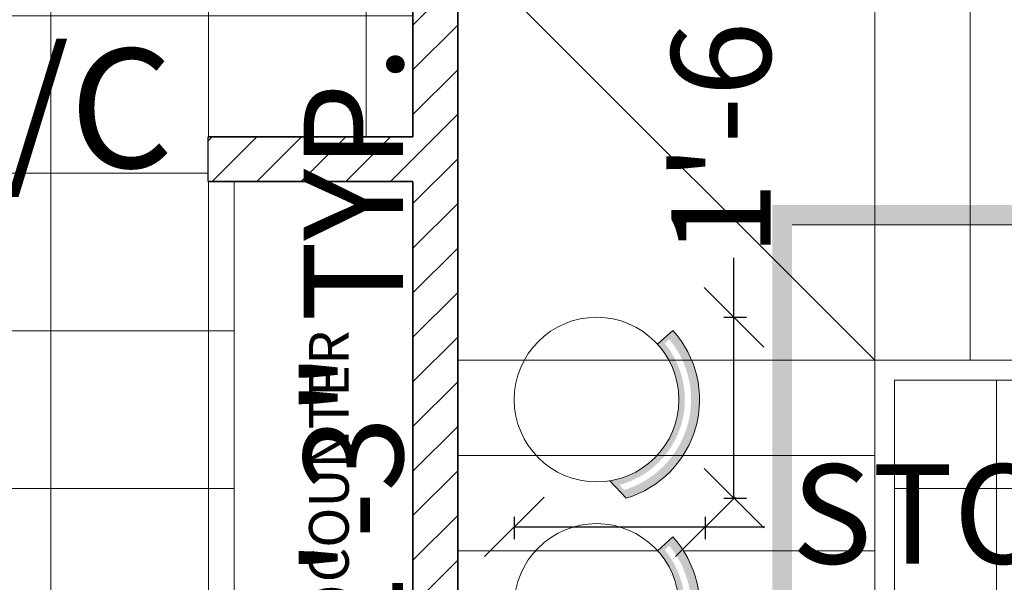
# Model space of a CAD drawing. Units: inches. Extents: x 2036 to 2670, y 319 to 920.
# Tile 9 of 15: x 2251 to 2350, y 784 to 841. Entities that reach past the tile are written whole.
import ezdxf

# ---------------------------------------------------------------- set-up
doc = ezdxf.new("R2010")
doc.units = ezdxf.units.IN
for name, color, linetype, lineweight in [('A-ANNO-DIMS', 2, 'Continuous', 18), ('A-ANNO-SYMB', 7, 'Continuous', 18), ('A-ANNO-SYMB-PATT', 7, 'Continuous', 13), ('A-ANNO-TEXT', 7, 'Continuous', 18), ('A-CASE', 7, 'Continuous', 18), ('A-DOOR', 3, 'Continuous', 25), ('A-FLOR-PATT', 8, 'Continuous', 9), ('A-FLOR-STRS', 7, 'Continuous', 18), ('A-FURN', 8, 'Continuous', 18), ('A-WALL', 7, 'Continuous', 35)]:
    doc.layers.add(name, color=color, linetype=linetype, lineweight=lineweight)
doc.layers.add('A-FURN-PATT', color=242, linetype='Continuous', lineweight=9, true_color=0xcd2027)
doc.layers.add('A-WALL-PATT', color=52, linetype='Continuous', lineweight=13, true_color=0xc8c92d)
doc.styles.get("Standard").update_dxf_attribs({"font": 'arial.ttf'})
doc.dimstyles.new('ISO-25', dxfattribs={"dimtxt": 10, "dimasz": 6, "dimexe": 1.25, "dimexo": 0.625, "dimtad": 0, "dimdec": 1, "dimlunit": 3, "dimtxsty": 'Standard', "dimblk": 'OBLIQUE', "dimcen": 2.5, "dimclrd": 94, "dimclre": 94, "dimclrt": 1, "dimadec": 0, "dimazin": 0, "dimtfac": 1, "dimtdec": 1, "dimtmove": 0, "dimatfit": 3, "dimfxl": 1, "dimfxlon": 1, "dimarcsym": 0})

# ---------------------------------------------------------------- blocks, each defined once
blk = doc.blocks.new('STOOL-COUNTER')
for p, q in [((14.44209721263451, 15.49845302218841), (15.97906463249819, 16.89025742639614)), ((16.25127518254248, 16.57729449613657), (16.25742551333951, 16.5828639424235)), ((9.61939974663892, 1.743797943406207), (11.27062915654505, 0.0001860092081643))]:
    blk.add_line(p, q)
blk.add_circle((8.294227533182038, 9.93123540535771), 8.29398659202474)
blk.add_arc((8.294227533182038, 9.93123540535771), 10.36748324003093, 286.6838234776646, 42.16248726182812)
blk = doc.blocks.new('_Oblique')
at = {"color": 0, "linetype": 'ByBlock', "lineweight": -2}
blk.add_line((-0.5, -0.5), (0.5, 0.5), dxfattribs=at)
blk = doc.blocks.new('*D23')
at = {"layer": 'A-ANNO-DIMS', "color": 94, "lineweight": -2, "transparency": 16777216}
for p, q in [((2286.028582728119, 660.1846446428973), (2286.028582728119, 666.1846446428973)), ((2285.02858272812, 660.1846446428973), (2287.27858272812, 660.1846446428973)), ((2286.028582728119, 633.1846547235), (2286.028582728119, 660.1846446428973)), ((2285.02858272812, 633.1846547235), (2287.27858272812, 633.1846547235))]:
    blk.add_line(p, q, dxfattribs=at)
at = {"layer": 'Defpoints', "color": 0, "transparency": 16777216}
for p in [(2281.978584240209, 660.1846446428973), (2286.028582728119, 660.1846446428973), (2281.978584240209, 633.1846547235)]:
    blk.add_point(p, dxfattribs=at)
at = {"layer": 'A-ANNO-DIMS', "color": 94, "lineweight": -2, "transparency": 16777216, "xscale": 6, "yscale": 6, "zscale": 6}
for p, rotation in [((2286.028582728119, 660.1846446428973), 90), ((2286.028582728119, 633.1846547235), 270)]:
    blk.add_blockref('_Oblique', p, dxfattribs=dict(at, rotation=rotation))
at = {"layer": 'A-ANNO-DIMS', "color": 1, "transparency": 16777216, "insert": (2286.028582728119, 755.2407496906455), "char_height": 10, "attachment_point": 5, "rotation": 90}
blk.add_mtext('ROCKING CHAIR 2\'-3" TYP.', dxfattribs=at)
blk = doc.blocks.new('*D27')
at = {"layer": 'A-ANNO-DIMS', "color": 94, "lineweight": -2, "transparency": 16777216}
for p, q in [((2300.931240941157, 790.9031204416938), (2300.931240941157, 788.6531204416938)), ((2320.167405879669, 790.9031204416938), (2320.167405879669, 788.6531204416938)), ((2300.931240941157, 789.9031204416937), (2320.167405879669, 789.9031204416937)), ((2320.167405879669, 789.9031204416937), (2326.167405879669, 789.9031204416937))]:
    blk.add_line(p, q, dxfattribs=at)
at = {"layer": 'Defpoints', "color": 0, "transparency": 16777216}
for p in [(2300.931240941157, 792.7885451824704), (2320.167405879669, 792.7885451824704), (2320.167405879669, 789.9031204416937)]:
    blk.add_point(p, dxfattribs=at)
at = {"layer": 'A-ANNO-DIMS', "color": 94, "lineweight": -2, "transparency": 16777216, "xscale": 6, "yscale": 6, "zscale": 6, "rotation": 180}
blk.add_blockref('_Oblique', (2300.931240941157, 789.9031204416937), dxfattribs=at)
at = {"layer": 'A-ANNO-DIMS', "color": 94, "lineweight": -2, "transparency": 16777216, "xscale": 6, "yscale": 6, "zscale": 6}
blk.add_blockref('_Oblique', (2320.167405879669, 789.9031204416937), dxfattribs=at)
at = {"layer": 'A-ANNO-DIMS', "color": 1, "transparency": 16777216, "insert": (2382.86334721664, 789.9031204416937), "char_height": 10, "attachment_point": 5}
blk.add_mtext('STOOL 1\'-7" TYP.', dxfattribs=at)
blk = doc.blocks.new('*D28')
at = {"layer": 'A-ANNO-DIMS', "color": 94, "lineweight": -2, "transparency": 16777216}
for p, q in [((2323.052830620447, 811.0135811706456), (2323.052830620447, 817.0135811706456)), ((2322.052830620447, 811.0135811706456), (2324.302830620447, 811.0135811706456)), ((2323.052830620447, 792.7885451824709), (2323.052830620447, 811.0135811706456)), ((2322.052830620447, 792.7885451824709), (2324.302830620447, 792.7885451824709))]:
    blk.add_line(p, q, dxfattribs=at)
at = {"layer": 'Defpoints', "color": 0, "transparency": 16777216}
for p in [(2320.167405879669, 811.0135811706456), (2323.052830620447, 811.0135811706456), (2320.167405879669, 792.7885451824709)]:
    blk.add_point(p, dxfattribs=at)
at = {"layer": 'A-ANNO-DIMS', "color": 94, "lineweight": -2, "transparency": 16777216, "xscale": 6, "yscale": 6, "zscale": 6}
for p, rotation in [((2323.052830620447, 811.0135811706456), 90), ((2323.052830620447, 792.7885451824709), 270)]:
    blk.add_blockref('_Oblique', p, dxfattribs=dict(at, rotation=rotation))
at = {"layer": 'A-ANNO-DIMS', "color": 1, "transparency": 16777216, "insert": (2323.052830620447, 847.6454024530459), "char_height": 10, "attachment_point": 5, "rotation": 90}
blk.add_mtext('1\'-6" TYP.', dxfattribs=at)
blk = doc.blocks.new('*D58')
at = {"layer": 'A-ANNO-DIMS', "color": 94, "lineweight": -2, "transparency": 16777216}
for p, q in [((2224.735119, 436.334645), (2224.735119, 434.0846449999999)), ((2270.113432, 436.334645), (2270.113432, 434.0846449999999)), ((2224.735119, 435.334645), (2270.113432, 435.334645)), ((2270.113432, 435.334645), (2276.113432, 435.334645))]:
    blk.add_line(p, q, dxfattribs=at)
at = {"layer": 'Defpoints', "color": 0, "transparency": 16777216}
for p in [(2224.735119, 824.684645), (2270.113432, 824.684645), (2270.113432, 435.334645)]:
    blk.add_point(p, dxfattribs=at)
at = {"layer": 'A-ANNO-DIMS', "color": 94, "lineweight": -2, "transparency": 16777216, "xscale": 6, "yscale": 6, "zscale": 6, "rotation": 180}
blk.add_blockref('_Oblique', (2224.735119, 435.334645), dxfattribs=at)
at = {"layer": 'A-ANNO-DIMS', "color": 94, "lineweight": -2, "transparency": 16777216, "xscale": 6, "yscale": 6, "zscale": 6}
blk.add_blockref('_Oblique', (2270.113432, 435.334645), dxfattribs=at)
at = {"layer": 'A-ANNO-DIMS', "color": 1, "transparency": 16777216, "insert": (2301.677040458391, 435.334645), "char_height": 10, "attachment_point": 5}
blk.add_mtext('3\'-9 1/2"', dxfattribs=at)

msp = doc.modelspace()

# ---------------------------------------------------------------- hatches: boundary and pattern name
at = {"layer": 'A-ANNO-SYMB-PATT'}
h = msp.add_hatch(color=256, dxfattribs=at)
h.dxf.hatch_style = 1
h.paths.add_polyline_path([(2406.873099182944, 822.3319931427415), (2326.913490001141, 822.3319931427415), (2326.913490001141, 772.4185847172232), (2322.238393735226, 772.4185847172232), (2328.913490001141, 764.3321655646498), (2328.913490001141, 772.4185847172232), (2328.913490001141, 820.3319931427413), (2404.873099182943, 820.3319931427413), (2404.873099182944, 731.1997691085871), (2406.873099182944, 731.1997691085871)])
at = {"layer": 'A-FLOR-PATT'}
h = msp.add_hatch(dxfattribs=at)
h.set_pattern_fill('ANSI31', color=256, scale=5, angle=135)
h.set_pattern_definition([(180, (0, 0), (-1.8e-15, -15.875), [])])
h.paths.add_polyline_path([(2290.73511852215, 659.6846447234993), (2158.73511852215, 659.6846447234993), (2158.73511852215, 582.5347262125274), (2158.73511852215, 545.5097979180838), (2158.73511852215, 503.6846447234993), (2426.735118522151, 503.6846447234993), (2426.735118522151, 614.6846447234993), (2426.735118522151, 623.6846447234993), (2426.735118522151, 628.1846447234993), (2431.235118522151, 628.1846447234993), (2431.235118522151, 623.6846447234993), (2438.735118522151, 623.6846447234993), (2438.735118522151, 619.1846447234993), (2574.394321277629, 619.1846447234993), (2574.394321277629, 623.7052101185), (2586.394321277629, 623.7052101185), (2586.394321277629, 619.1846447234993), (2603.735118522151, 619.1846447234993), (2603.735118522151, 824.6846447234993), (2431.73511852215, 824.6846447234993), (2431.73511852215, 746.0911818027907), (2439.235118522151, 746.0911818027907), (2439.235118522151, 737.0911818027907), (2431.73511852215, 737.0911818027907), (2431.73511852215, 659.6846447234992), (2427.235118522151, 659.6846447234992), (2427.235118522151, 739.4846447234991), (2383.235118522151, 739.4846447234991), (2383.23511852215, 804.6846447234994), (2339.235118522151, 804.6846447234994), (2339.235118522151, 749.0846447234992), (2295.235118522151, 749.084644723499), (2295.235118522151, 737.6459187756934), (2295.267038589669, 737.6459187756934), (2295.267038589669, 728.6459187756934), (2295.213454263402, 728.6459187756934, -0.5864181262682077), (2272.735118522151, 728.6846447234993), (2272.735118522151, 824.6846447234994), (2270.11343239043, 824.6846447234994), (2270.11343239043, 829.1846447234994), (2290.73511852215, 829.1846447234993), (2290.73511852215, 848.663139280863), (2283.207837384491, 848.663139280863), (2283.207837384491, 857.663139280863), (2289.735118522151, 857.663139280863), (2289.735118522151, 874.6846447234994), (2158.73511852215, 874.6846447234993), (2158.73511852215, 852.8142946291669), (2161.73511852215, 852.8142946291669), (2161.73511852215, 843.8142946291669), (2158.73511852215, 843.8142946291669), (2158.73511852215, 829.1846447234993), (2224.73511852215, 829.1846447234993), (2224.73511852215, 800.6846447234994), (2182.735118522151, 800.6846447234994), (2182.735118522151, 733.4146909245898), (2158.73511852215, 733.4146909245898), (2158.73511852215, 728.6846447234993), (2235.235118522151, 728.6846447234993), (2235.235118522151, 714.8073923633797), (2230.735118522151, 714.8073923633797), (2230.735118522151, 724.1846447234991), (2158.73511852215, 724.1846447234993), (2158.73511852215, 664.1846447234993), (2230.735118522151, 664.1846447234993), (2230.735118522151, 678.8073923633796), (2235.235118522151, 678.8073923633796), (2235.235118522151, 664.1846447234993), (2290.73511852215, 664.1846447234993)])
h.paths.add_polyline_path([(2309.267682807548, 612.1195713103912), (2309.267682807548, 603.1195713103912), (2297.267682807548, 603.1195713103912), (2297.267682807548, 612.1195713103912)], flags=16)
h.paths.add_polyline_path([(2280.116432231614, 639.1101421987634), (2280.261038064034, 638.1846547234999, -0.4142135623730951), (2279.261038064034, 637.1846547234999), (2278.761038064034, 637.1846547234999), (2279.261038064034, 633.1846547234999), (2277.761038064034, 633.1846547234999), (2277.261038064034, 637.1846547234999), (2269.761038064034, 637.1846547234999), (2262.261038064034, 637.1846547234999), (2261.761038064034, 633.1846547234999), (2260.261038064034, 633.1846547234999), (2260.761038064034, 637.1846547234999), (2260.261038064034, 637.1846547234999, -0.4142135623730951), (2259.261038064034, 638.1846547234999), (2259.405649624543, 639.1101427248512, -0.5411643393254109), (2257.761038870006, 641.1846576787281), (2260.761038064034, 652.1846447234999), (2261.448547850994, 652.1846447234999), (2261.52666276384, 652.6846447234999), (2262.761038064034, 652.6846447234999), (2262.249174101338, 655.2439645369782, 0.0019132646615086), (2261.761062671999, 655.1846078115532), (2259.76103814896, 658.1846445961108, -0.1500000140127399), (2279.761037979108, 658.184644596111), (2277.761013456069, 655.1846078115531, 0.0019132646615084), (2277.27290202673, 655.243964536978), (2276.761038064034, 652.6846447234999), (2277.995414002001, 652.6846447234999), (2278.073538681693, 652.1846447234999), (2278.761038064034, 652.1846447234999), (2281.761037258062, 641.1846576787256, -0.5411631634674846)], flags=16)
h.paths.add_polyline_path([(2245.983724681685, 639.1101421987634), (2246.128330514105, 638.1846547234998, -0.4142135623730951), (2245.128330514105, 637.1846547234996), (2244.628330514105, 637.1846547234996), (2245.128330514105, 633.1846547234996), (2243.628330514105, 633.1846547234996), (2243.128330514105, 637.1846547234996), (2235.628330514105, 637.1846547234996), (2228.128330514104, 637.1846547234996), (2227.628330514105, 633.1846547234996), (2226.128330514105, 633.1846547234996), (2226.628330514105, 637.1846547234996), (2226.128330514105, 637.1846547234996, -0.4142135623730951), (2225.128330514105, 638.1846547234998), (2225.272942074614, 639.1101427248511, -0.5411643393254109), (2223.628331320076, 641.184657678728), (2226.628330514105, 652.1846447234998), (2227.315840301064, 652.1846447234998), (2227.393955213911, 652.6846447234998), (2228.628330514105, 652.6846447234998), (2228.116466551409, 655.243964536978, 0.0019132646615086), (2227.628355122069, 655.1846078115532), (2225.628330599031, 658.1846445961108, -0.1500000140127405), (2245.628330429179, 658.1846445961108), (2243.62830590614, 655.184607811553, 0.0019132646615084), (2243.140194476801, 655.2439645369778), (2242.628330514105, 652.6846447234998), (2243.862706452072, 652.6846447234998), (2243.940831131764, 652.1846447234998), (2244.628330514105, 652.1846447234998), (2247.628329708133, 641.1846576787256, -0.5411631634675002)], flags=16)
h.paths.add_polyline_path([(2351.589714523122, 515.1547705889745, -0.151947809280591), (2279.589707523122, 515.1547621898734), (2279.589707523122, 537.684644723502), (2273.589707523122, 537.684644723502), (2273.589707523122, 511.6846368176175, 0.1904762075443491), (2357.589714523122, 511.6846553964427), (2357.589714523122, 537.684644723502), (2351.589714523122, 537.684644723502)])
h.paths.add_polyline_path([(2327.589707523122, 536.1267447235019), (2327.589714897934, 517.0665447235019), (2303.58971014831, 517.0665447235019), (2303.589717523122, 536.1267447235019)], flags=16)
h.paths.add_polyline_path([(2213.4008319258, 639.1101421987634), (2213.545437758219, 638.1846547234998, -0.4142135623730951), (2212.545437758219, 637.1846547234996), (2212.045437758219, 637.1846547234996), (2212.545437758219, 633.1846547234996), (2211.045437758219, 633.1846547234996), (2210.545437758219, 637.1846547234996), (2203.045437758219, 637.1846547234996), (2195.545437758219, 637.1846547234996), (2195.045437758219, 633.1846547234996), (2193.545437758219, 633.1846547234996), (2194.045437758219, 637.1846547234996), (2193.545437758219, 637.1846547234996, -0.4142135623730951), (2192.545437758219, 638.1846547234998), (2192.690049318728, 639.1101427248511, -0.5411643393254677), (2191.045438564191, 641.1846576787283), (2194.045437758219, 652.1846447234998), (2194.732947545178, 652.1846447234998), (2194.811062458025, 652.6846447234998), (2196.045437758219, 652.6846447234998), (2195.533573795524, 655.243964536978, 0.0019132646615086), (2195.045462366184, 655.1846078115532), (2193.045437843145, 658.1846445961108, -0.1500000140127405), (2213.045437673293, 658.1846445961108), (2211.045413150255, 655.184607811553, 0.0019132646615084), (2210.557301720915, 655.2439645369778), (2210.045437758219, 652.6846447234998), (2211.279813696187, 652.6846447234998), (2211.357938375878, 652.1846447234998), (2212.045437758219, 652.1846447234998), (2215.045436952248, 641.1846576787256, -0.541163163467504)], flags=16)
h.paths.add_polyline_path([(2368.579245727136, 538.0174860170698), (2370.522614835591, 538.0174860170698), (2371.170404538409, 532.8351683945237), (2380.887250080682, 532.8351683945237), (2390.604095622956, 532.8351683945237), (2391.251885325774, 538.0174860170698), (2393.195254434229, 538.0174860170698), (2392.547464731411, 532.8351683945237), (2380.887250080682, 532.8351683945237), (2368.579245727136, 532.8351683945237, 0.4142135623730823), (2367.283666321499, 531.5395889888874), (2367.471014659917, 530.3405464757611, -0.4833518268794939), (2369.227035511853, 527.6528503215334), (2371.818194241227, 513.4014902657708), (2370.117745471103, 513.4014902657708), (2370.218962197183, 512.7537005629525), (2391.555537137895, 512.7537005629525), (2391.656741210253, 513.4014902657708), (2389.956305920138, 513.4014902657708), (2392.547464649512, 527.6528503215332, -1.387427444475197), (2396.43420190412, 527.6528469432474), (2392.547464731411, 513.4014902657708), (2391.656741210253, 513.4014902657708), (2391.555537137895, 512.7537005629525), (2389.30851621732, 512.7537005629525), (2389.996735292977, 509.3669642787241, 0.003795645225288), (2391.251853444202, 509.5147998712193), (2393.843044027018, 505.6280139969943, -0.1500000140127354), (2367.931456134346, 505.6280139969944), (2370.522646717163, 509.5147998712195, 0.0039006605371613), (2371.812521455224, 509.3631450934526), (2372.465983944045, 512.7537005629525), (2370.218962197183, 512.7537005629525), (2370.117745471103, 513.4014902657708), (2369.227035429954, 513.4014902657708), (2365.340298257246, 527.6528469432453, -0.5411631634679974), (2367.471014659917, 530.3405464757611), (2367.283666321499, 531.5395889888874, -0.4142135623730824), (2368.579245727136, 532.8351683945237), (2369.227035429954, 532.8351683945237)])
h.paths.add_polyline_path([(2266.737911501414, 538.0174860170694), (2266.090121798596, 532.8351683945236), (2254.429907147867, 532.8351683945236), (2242.121902794321, 532.8351683945235, 0.4142135623730823), (2240.826323388684, 531.539588988887), (2241.013671727102, 530.3405464757608, -0.4833518268795056), (2242.769692579038, 527.652850321533), (2245.360851308412, 513.4014902657705), (2243.660402538288, 513.4014902657705), (2243.761619264368, 512.7537005629522), (2265.09819420508, 512.7537005629522), (2265.199398277438, 513.4014902657703), (2263.498962987323, 513.4014902657703), (2266.090121716697, 527.6528503215327, -1.387427444474997), (2269.976858971305, 527.6528469432478), (2266.090121798596, 513.4014902657703), (2265.199398277438, 513.4014902657703), (2265.09819420508, 512.7537005629522), (2262.851173284504, 512.7537005629522), (2263.539392360161, 509.3669642787239, 0.0037956452252879), (2264.794510511388, 509.5147998712191), (2267.385701094204, 505.628013996994, -0.1500000140127357), (2241.474113201531, 505.6280139969941), (2244.065303784347, 509.5147998712193, 0.0039006605371612), (2245.355178522409, 509.3631450934523), (2246.00864101123, 512.7537005629522), (2243.761619264368, 512.7537005629522), (2243.660402538288, 513.4014902657705), (2242.769692497139, 513.4014902657705), (2238.88295532443, 527.6528469432458, -0.541163163467894), (2241.013671727102, 530.3405464757608), (2240.826323388684, 531.539588988887, -0.4142135623730824), (2242.121902794321, 532.8351683945235), (2242.769692497139, 532.8351683945235), (2242.121902794321, 538.0174860170694), (2244.065271902775, 538.0174860170694), (2244.713061605594, 532.8351683945236), (2254.429907147867, 532.8351683945236), (2264.146752690141, 532.8351683945236), (2264.794542392959, 538.0174860170694)])
h.paths.add_polyline_path([(2185.23510852215, 620.3554545661904), (2185.23510852215, 618.8554545661904), (2181.23510852215, 618.3554545661904), (2181.23510852215, 610.8554545661904), (2181.23510852215, 603.3554545661904), (2185.23510852215, 602.8554545661904), (2185.23510852215, 601.3554545661905), (2181.23510852215, 601.8554545661904), (2181.23510852215, 601.3554545661905, -0.4142135623730951), (2180.23510852215, 600.3554545661905), (2179.309620520799, 600.5000661266993, -0.5411643393248329), (2177.235105566925, 598.8554553721619), (2166.23511852215, 601.8554545661904), (2166.23511852215, 602.5429643531498), (2165.73511852215, 602.6210792659967), (2165.73511852215, 603.8554545661904), (2163.175798708671, 603.3435906034947, 0.0019132646615093), (2163.235155434097, 602.8554791741547), (2160.235118649539, 600.8554546511162, -0.1500000140127393), (2160.235118649539, 620.8554544812645), (2163.235155434097, 618.855429958226, 0.0019132646615086), (2163.175798708672, 618.3673185288861), (2165.73511852215, 617.8554545661905), (2165.73511852215, 619.0898305041582), (2166.23511852215, 619.167955183849), (2166.23511852215, 619.8554545661904), (2177.235105566925, 622.855453760219, -0.5411631634675461), (2179.309621046886, 621.2108487337705), (2180.23510852215, 621.3554545661905, -0.4142135623730951), (2181.23510852215, 620.3554545661904), (2181.23510852215, 619.8554545661904)])
h.paths.add_polyline_path([(2470.924455674587, 676.0076055808825), (2470.924455674587, 806.1287861477749), (2568.515288238047, 806.1287861477749), (2568.515288238047, 676.0076055808825)], flags=16)
h.paths.add_polyline_path([(2177.737763186158, 677.4877546326836), (2161.903034523561, 677.4877546326836), (2161.903034523561, 705.8482879805396), (2177.737763186158, 705.8482879805396)], flags=16)
h.paths.add_polyline_path([(2176.737763186158, 678.4877546326836), (2162.903034523562, 678.4877546326836), (2162.903034523562, 704.8482879805395), (2176.737763186158, 704.8482879805395)], flags=0)
h.paths.add_polyline_path([(2175.006477017632, 686.4819431438401), (2172.932045752523, 686.4819431438401), (2172.932045752523, 690.6308056740573), (2170.857614487415, 690.6308056740573), (2170.857614487415, 686.4819431438401), (2164.634320692089, 686.4819431438401), (2164.634320692089, 688.556374408949), (2166.708751957198, 688.5563744089487), (2168.783183222306, 688.5563744089487), (2168.783183222306, 690.6308056740573), (2164.634320692089, 690.6308056740575), (2164.634320692089, 696.8540994693836), (2166.708751957198, 696.8540994693833), (2166.708751957198, 692.7052369391664), (2168.783183222306, 692.7052369391664), (2168.783183222306, 696.8540994693833), (2175.006477017632, 696.8540994693833), (2175.006477017632, 694.7796682042747), (2170.857614487415, 694.7796682042747), (2170.857614487415, 692.705236939166), (2175.006477017632, 692.705236939166)], flags=0)
h.paths.add_polyline_path([(2543.792289466609, 782.7069824289107), (2483.936552586593, 782.7069824289107), (2483.936552586593, 804.1769691712028), (2517.768030582033, 804.1769691712028), (2517.768030582033, 782.7069824289107), (2521.671680800318, 782.7069824289107), (2521.671680800318, 804.1769691712028), (2555.5031750609, 804.1769691712028), (2555.5031750609, 779.4539541346239), (2547.045315620746, 779.4539541346239), (2568.515288238047, 757.9839673923317), (2543.792289466609, 757.9839673923317)], flags=0)
h.paths.add_polyline_path([(2584.586509881755, 727.592712465714), (2584.586509881755, 736.592712465714), (2596.586509881755, 736.592712465714), (2596.586509881755, 727.592712465714)], flags=16)
h.paths.add_polyline_path([(2520.447962588816, 647.0347442731018), (2553.787662452391, 647.0347442731018), (2553.787662452391, 658.2291508215328), (2520.447962588816, 658.2291508215328)], flags=24)
h.paths.add_polyline_path([(2299.532438080047, 573.74198835745), (2331.707745037755, 573.74198835745), (2331.707745037755, 584.9363949058811), (2299.532438080047, 584.9363949058811)], flags=24)
h.paths.add_polyline_path([(2191.59306945766, 685.1871821201288), (2212.116261817823, 685.1871821201288), (2212.116261817823, 696.3815886685599), (2191.59306945766, 696.3815886685599)], flags=24)
h.paths.add_polyline_path([(2353.895364950782, 649.8625097966332), (2379.080221703851, 649.8625097966332), (2379.080221703851, 661.0569163450643), (2353.895364950782, 661.0569163450643)], flags=24)
h.paths.add_polyline_path([(2214.607247066254, 763.3108194044448), (2237.461271622871, 763.3108194044448), (2237.461271622871, 779.5563855708841), (2214.607247066254, 779.5563855708841)], flags=24)
h.paths.add_polyline_path([(2225.093254720334, 819.3065323559471), (2269.286979140525, 819.3065323559471), (2269.286979140525, 844.0350453163835), (2225.093254720334, 844.0350453163835)], flags=24)
h.paths.add_polyline_path([(2204.061908777108, 845.0427705104745), (2226.915933333724, 845.0427705104745), (2226.915933333724, 856.2371770589056), (2204.061908777108, 856.2371770589056)], flags=24)
h = msp.add_hatch(dxfattribs=at)
h.set_pattern_fill('ANSI31', color=256, scale=5, angle=45)
h.set_pattern_definition([(90, (0, 0), (-15.875, 0), [])])
h.paths.add_polyline_path([(2290.73511852215, 659.6846447234993), (2158.73511852215, 659.6846447234993), (2158.73511852215, 582.5347262125274), (2158.73511852215, 545.5097979180838), (2158.73511852215, 503.6846447234993), (2426.735118522151, 503.6846447234993), (2426.735118522151, 614.6846447234993), (2426.735118522151, 623.6846447234993), (2426.735118522151, 628.1846447234993), (2431.235118522151, 628.1846447234993), (2431.235118522151, 623.6846447234993), (2438.735118522151, 623.6846447234993), (2438.735118522151, 619.1846447234993), (2574.394321277629, 619.1846447234993), (2574.394321277629, 623.7052101185), (2586.394321277629, 623.7052101185), (2586.394321277629, 619.1846447234993), (2603.735118522151, 619.1846447234993), (2603.735118522151, 824.6846447234993), (2431.73511852215, 824.6846447234993), (2431.73511852215, 746.0911818027907), (2439.235118522151, 746.0911818027907), (2439.235118522151, 737.0911818027907), (2431.73511852215, 737.0911818027907), (2431.73511852215, 659.6846447234992), (2427.235118522151, 659.6846447234992), (2427.235118522151, 739.4846447234991), (2383.235118522151, 739.4846447234991), (2383.23511852215, 804.6846447234994), (2339.235118522151, 804.6846447234994), (2339.235118522151, 749.0846447234992), (2295.235118522151, 749.084644723499), (2295.235118522151, 737.6459187756934), (2295.267038589669, 737.6459187756934), (2295.267038589669, 728.6459187756934), (2295.213454263402, 728.6459187756934, -0.5864181262682077), (2272.735118522151, 728.6846447234993), (2272.735118522151, 824.6846447234994), (2270.11343239043, 824.6846447234994), (2270.11343239043, 829.1846447234994), (2290.73511852215, 829.1846447234993), (2290.73511852215, 848.663139280863), (2283.207837384491, 848.663139280863), (2283.207837384491, 857.663139280863), (2289.735118522151, 857.663139280863), (2289.735118522151, 874.6846447234994), (2158.73511852215, 874.6846447234993), (2158.73511852215, 852.8142946291669), (2161.73511852215, 852.8142946291669), (2161.73511852215, 843.8142946291669), (2158.73511852215, 843.8142946291669), (2158.73511852215, 829.1846447234993), (2224.73511852215, 829.1846447234993), (2224.73511852215, 800.6846447234994), (2182.735118522151, 800.6846447234994), (2182.735118522151, 733.4146909245898), (2158.73511852215, 733.4146909245898), (2158.73511852215, 728.6846447234993), (2235.235118522151, 728.6846447234993), (2235.235118522151, 714.8073923633797), (2230.735118522151, 714.8073923633797), (2230.735118522151, 724.1846447234991), (2158.73511852215, 724.1846447234993), (2158.73511852215, 664.1846447234993), (2230.735118522151, 664.1846447234993), (2230.735118522151, 678.8073923633796), (2235.235118522151, 678.8073923633796), (2235.235118522151, 664.1846447234993), (2290.73511852215, 664.1846447234993)])
h.paths.add_polyline_path([(2309.267682807548, 612.1195713103912), (2309.267682807548, 603.1195713103912), (2297.267682807548, 603.1195713103912), (2297.267682807548, 612.1195713103912)], flags=16)
h.paths.add_polyline_path([(2280.116432231614, 639.1101421987635), (2280.261038064034, 638.1846547234999, -0.4142135623730951), (2279.261038064034, 637.1846547234999), (2278.761038064034, 637.1846547234999), (2279.261038064034, 633.1846547234999), (2277.761038064034, 633.1846547234999), (2277.261038064034, 637.1846547234999), (2269.761038064034, 637.1846547234999), (2262.261038064034, 637.1846547234999), (2261.761038064034, 633.1846547234999), (2260.261038064034, 633.1846547234999), (2260.761038064034, 637.1846547234999), (2260.261038064034, 637.1846547234999, -0.414213562373095), (2259.261038064034, 638.1846547234999), (2259.405649624543, 639.1101427248512, -0.5411643393254109), (2257.761038870006, 641.1846576787281), (2260.761038064034, 652.1846447234999), (2261.448547850994, 652.1846447234999), (2261.52666276384, 652.6846447234999), (2262.761038064034, 652.6846447234999), (2262.249174101338, 655.2439645369782, 0.0019132646615086), (2261.761062671999, 655.1846078115532), (2259.76103814896, 658.1846445961108, -0.1500000140127399), (2279.761037979108, 658.184644596111), (2277.761013456069, 655.1846078115531, 0.0019132646615085), (2277.27290202673, 655.243964536978), (2276.761038064034, 652.6846447234999), (2277.995414002001, 652.6846447234999), (2278.073538681693, 652.1846447234999), (2278.761038064034, 652.1846447234999), (2281.761037258062, 641.1846576787257, -0.5411631634675018)], flags=16)
h.paths.add_polyline_path([(2245.983724681685, 639.1101421987634), (2246.128330514105, 638.1846547234998, -0.4142135623730951), (2245.128330514105, 637.1846547234996), (2244.628330514105, 637.1846547234996), (2245.128330514105, 633.1846547234996), (2243.628330514105, 633.1846547234996), (2243.128330514105, 637.1846547234996), (2235.628330514105, 637.1846547234996), (2228.128330514104, 637.1846547234996), (2227.628330514105, 633.1846547234996), (2226.128330514105, 633.1846547234996), (2226.628330514105, 637.1846547234996), (2226.128330514105, 637.1846547234996, -0.414213562373095), (2225.128330514105, 638.1846547234998), (2225.272942074614, 639.1101427248511, -0.5411643393254109), (2223.628331320076, 641.184657678728), (2226.628330514105, 652.1846447234998), (2227.315840301064, 652.1846447234998), (2227.393955213911, 652.6846447234998), (2228.628330514105, 652.6846447234998), (2228.116466551409, 655.243964536978, 0.0019132646615086), (2227.628355122069, 655.1846078115532), (2225.628330599031, 658.1846445961108, -0.1500000140127405), (2245.628330429179, 658.1846445961108), (2243.62830590614, 655.184607811553, 0.0019132646615084), (2243.140194476801, 655.2439645369778), (2242.628330514105, 652.6846447234998), (2243.862706452072, 652.6846447234998), (2243.940831131764, 652.1846447234998), (2244.628330514105, 652.1846447234998), (2247.628329708133, 641.1846576787256, -0.5411631634675091)], flags=16)
h.paths.add_polyline_path([(2351.589714523122, 537.684644723502), (2351.589714523122, 515.1547705889745, -0.151947809280591), (2279.589707523122, 515.1547621898734), (2279.589707523122, 537.684644723502), (2273.589707523122, 537.684644723502), (2273.589707523122, 511.6846368176175, 0.1904762075443491), (2357.589714523122, 511.6846553964427), (2357.589714523122, 537.684644723502)])
h.paths.add_polyline_path([(2368.579245727136, 538.0174860170698), (2370.522614835591, 538.0174860170698), (2371.170404538409, 532.8351683945237), (2380.887250080682, 532.8351683945237), (2390.604095622956, 532.8351683945237), (2391.251885325774, 538.0174860170698), (2393.195254434229, 538.0174860170698), (2392.547464731411, 532.8351683945237), (2380.887250080682, 532.8351683945237), (2368.579245727136, 532.8351683945237, 0.4142135623730823), (2367.283666321499, 531.5395889888874), (2367.471014659917, 530.3405464757611, -0.4833518268794933), (2369.227035511853, 527.6528503215334), (2371.818194241227, 513.4014902657708), (2370.117745471103, 513.4014902657708), (2370.218962197183, 512.7537005629525), (2391.555537137895, 512.7537005629525), (2391.656741210253, 513.4014902657708), (2389.956305920138, 513.4014902657708), (2392.547464649512, 527.6528503215332, -1.387427444475181), (2396.43420190412, 527.6528469432474), (2392.547464731411, 513.4014902657708), (2391.656741210253, 513.4014902657708), (2391.555537137895, 512.7537005629525), (2389.30851621732, 512.7537005629525), (2389.996735292977, 509.3669642787241, 0.003795645225288), (2391.251853444202, 509.5147998712193), (2393.843044027018, 505.6280139969943, -0.1500000140127354), (2367.931456134346, 505.6280139969944), (2370.522646717163, 509.5147998712195, 0.0039006605371613), (2371.812521455224, 509.3631450934526), (2372.465983944045, 512.7537005629525), (2370.218962197183, 512.7537005629525), (2370.117745471103, 513.4014902657708), (2369.227035429954, 513.4014902657708), (2365.340298257246, 527.6528469432453, -0.5411631634679983), (2367.471014659917, 530.3405464757611), (2367.283666321499, 531.5395889888874, -0.4142135623730824), (2368.579245727136, 532.8351683945237), (2369.227035429954, 532.8351683945237)])
h.paths.add_polyline_path([(2327.589707523122, 536.1267447235019), (2327.589714897934, 517.0665447235019), (2303.58971014831, 517.0665447235019), (2303.589717523122, 536.1267447235019)], flags=16)
h.paths.add_polyline_path([(2470.924455674587, 676.0076055808825), (2470.924455674587, 806.1287861477749), (2568.515288238047, 806.1287861477749), (2568.515288238047, 676.0076055808825)], flags=16)
h.paths.add_polyline_path([(2266.737911501414, 538.0174860170694), (2266.090121798596, 532.8351683945236), (2254.429907147867, 532.8351683945236), (2242.121902794321, 532.8351683945235, 0.4142135623730823), (2240.826323388684, 531.539588988887), (2241.013671727102, 530.3405464757608, -0.4833518268795056), (2242.769692579038, 527.652850321533), (2245.360851308412, 513.4014902657705), (2243.660402538288, 513.4014902657705), (2243.761619264368, 512.7537005629522), (2265.09819420508, 512.7537005629522), (2265.199398277438, 513.4014902657703), (2263.498962987323, 513.4014902657703), (2266.090121716697, 527.6528503215329, -1.38742744447494), (2269.976858971305, 527.6528469432479), (2266.090121798596, 513.4014902657703), (2265.199398277438, 513.4014902657703), (2265.09819420508, 512.7537005629522), (2262.851173284504, 512.7537005629522), (2263.539392360161, 509.3669642787239, 0.0037956452252879), (2264.794510511388, 509.5147998712191), (2267.385701094204, 505.628013996994, -0.1500000140127357), (2241.474113201531, 505.6280139969941), (2244.065303784347, 509.5147998712193, 0.0039006605371612), (2245.355178522409, 509.3631450934523), (2246.00864101123, 512.7537005629522), (2243.761619264368, 512.7537005629522), (2243.660402538288, 513.4014902657705), (2242.769692497139, 513.4014902657705), (2238.88295532443, 527.6528469432458, -0.5411631634678908), (2241.013671727102, 530.3405464757608), (2240.826323388684, 531.539588988887, -0.4142135623730824), (2242.121902794321, 532.8351683945235), (2242.769692497139, 532.8351683945235), (2242.121902794321, 538.0174860170694), (2244.065271902775, 538.0174860170694), (2244.713061605594, 532.8351683945236), (2254.429907147867, 532.8351683945236), (2264.146752690141, 532.8351683945236), (2264.794542392959, 538.0174860170694)])
h.paths.add_polyline_path([(2213.4008319258, 639.1101421987634), (2213.545437758219, 638.1846547234998, -0.4142135623730953), (2212.545437758219, 637.1846547234996), (2212.045437758219, 637.1846547234996), (2212.545437758219, 633.1846547234996), (2211.045437758219, 633.1846547234996), (2210.545437758219, 637.1846547234996), (2203.045437758219, 637.1846547234996), (2195.545437758219, 637.1846547234996), (2195.045437758219, 633.1846547234996), (2193.545437758219, 633.1846547234996), (2194.045437758219, 637.1846547234996), (2193.545437758219, 637.1846547234996, -0.414213562373095), (2192.545437758219, 638.1846547234998), (2192.690049318728, 639.1101427248511, -0.5411643393254677), (2191.045438564191, 641.1846576787283), (2194.045437758219, 652.1846447234998), (2194.732947545179, 652.1846447234998), (2194.811062458025, 652.6846447234998), (2196.045437758219, 652.6846447234998), (2195.533573795524, 655.243964536978, 0.0019132646615086), (2195.045462366184, 655.1846078115532), (2193.045437843145, 658.1846445961108, -0.1500000140127405), (2213.045437673293, 658.1846445961108), (2211.045413150255, 655.184607811553, 0.0019132646615084), (2210.557301720915, 655.2439645369778), (2210.045437758219, 652.6846447234998), (2211.279813696187, 652.6846447234998), (2211.357938375878, 652.1846447234998), (2212.045437758219, 652.1846447234998), (2215.045436952248, 641.1846576787254, -0.5411631634674544)], flags=16)
h.paths.add_polyline_path([(2185.23510852215, 620.3554545661904), (2185.23510852215, 618.8554545661904), (2181.23510852215, 618.3554545661904), (2181.23510852215, 610.8554545661904), (2181.23510852215, 603.3554545661904), (2185.23510852215, 602.8554545661904), (2185.23510852215, 601.3554545661905), (2181.23510852215, 601.8554545661904), (2181.23510852215, 601.3554545661905, -0.4142135623730951), (2180.23510852215, 600.3554545661905), (2179.309620520799, 600.5000661266993, -0.5411643393248329), (2177.235105566925, 598.8554553721619), (2166.23511852215, 601.8554545661904), (2166.23511852215, 602.5429643531498), (2165.73511852215, 602.6210792659967), (2165.73511852215, 603.8554545661904), (2163.175798708671, 603.3435906034947, 0.0019132646615093), (2163.235155434097, 602.8554791741547), (2160.235118649539, 600.8554546511162, -0.1500000140127393), (2160.235118649539, 620.8554544812645), (2163.235155434097, 618.855429958226, 0.0019132646615086), (2163.175798708672, 618.3673185288861), (2165.73511852215, 617.8554545661905), (2165.73511852215, 619.0898305041582), (2166.23511852215, 619.167955183849), (2166.23511852215, 619.8554545661904), (2177.235105566925, 622.855453760219, -0.5411631634675461), (2179.309621046886, 621.2108487337705), (2180.23510852215, 621.3554545661905, -0.4142135623730951), (2181.23510852215, 620.3554545661904), (2181.23510852215, 619.8554545661904)])
h.paths.add_polyline_path([(2177.737763186158, 677.4877546326836), (2161.903034523561, 677.4877546326836), (2161.903034523561, 705.8482879805396), (2177.737763186158, 705.8482879805396)], flags=16)
h.paths.add_polyline_path([(2176.737763186158, 678.4877546326836), (2162.903034523562, 678.4877546326836), (2162.903034523562, 704.8482879805395), (2176.737763186158, 704.8482879805395)], flags=0)
h.paths.add_polyline_path([(2175.006477017632, 686.4819431438401), (2172.932045752523, 686.4819431438401), (2172.932045752523, 690.6308056740573), (2170.857614487415, 690.6308056740573), (2170.857614487415, 686.4819431438401), (2164.634320692089, 686.4819431438401), (2164.634320692089, 688.556374408949), (2166.708751957198, 688.5563744089487), (2168.783183222306, 688.5563744089487), (2168.783183222306, 690.6308056740573), (2164.634320692089, 690.6308056740575), (2164.634320692089, 696.8540994693836), (2166.708751957198, 696.8540994693833), (2166.708751957198, 692.7052369391664), (2168.783183222306, 692.7052369391664), (2168.783183222306, 696.8540994693833), (2175.006477017632, 696.8540994693833), (2175.006477017632, 694.7796682042747), (2170.857614487415, 694.7796682042747), (2170.857614487415, 692.705236939166), (2175.006477017632, 692.705236939166)], flags=0)
h.paths.add_polyline_path([(2543.792289466609, 782.7069824289107), (2483.936552586593, 782.7069824289107), (2483.936552586593, 804.1769691712028), (2517.768030582033, 804.1769691712028), (2517.768030582033, 782.7069824289107), (2521.671680800318, 782.7069824289107), (2521.671680800318, 804.1769691712028), (2555.5031750609, 804.1769691712028), (2555.5031750609, 779.4539541346239), (2547.045315620746, 779.4539541346239), (2568.515288238047, 757.9839673923317), (2543.792289466609, 757.9839673923317)], flags=0)
h.paths.add_polyline_path([(2584.586509881755, 727.592712465714), (2584.586509881755, 736.592712465714), (2596.586509881755, 736.592712465714), (2596.586509881755, 727.592712465714)], flags=16)
h.paths.add_polyline_path([(2520.447962588816, 647.0347442731018), (2553.787662452391, 647.0347442731018), (2553.787662452391, 658.2291508215328), (2520.447962588816, 658.2291508215328)], flags=24)
h.paths.add_polyline_path([(2299.532438080047, 573.74198835745), (2331.707745037755, 573.74198835745), (2331.707745037755, 584.9363949058811), (2299.532438080047, 584.9363949058811)], flags=24)
h.paths.add_polyline_path([(2191.59306945766, 685.1871821201288), (2212.116261817823, 685.1871821201288), (2212.116261817823, 696.3815886685599), (2191.59306945766, 696.3815886685599)], flags=24)
h.paths.add_polyline_path([(2353.895364950782, 649.8625097966332), (2379.080221703851, 649.8625097966332), (2379.080221703851, 661.0569163450643), (2353.895364950782, 661.0569163450643)], flags=24)
h.paths.add_polyline_path([(2214.607247066254, 763.3108194044448), (2237.461271622871, 763.3108194044448), (2237.461271622871, 779.5563855708841), (2214.607247066254, 779.5563855708841)], flags=24)
h.paths.add_polyline_path([(2225.093254720334, 819.3065323559471), (2269.286979140525, 819.3065323559471), (2269.286979140525, 844.0350453163835), (2225.093254720334, 844.0350453163835)], flags=24)
h.paths.add_polyline_path([(2204.061908777108, 845.0427705104745), (2226.915933333724, 845.0427705104745), (2226.915933333724, 856.2371770589056), (2204.061908777108, 856.2371770589056)], flags=24)
at = {"layer": 'A-FURN-PATT'}
h = msp.add_hatch(color=256, dxfattribs=at)
h.dxf.hatch_style = 1
h.paths.add_polyline_path([(2316.910064632498, 809.678616599659), (2315.373097212635, 808.2868121954515, -0.0594262793657001), (2316.510046744205, 806.6846447234993), (2317.181130003143, 806.6846447234993, 0.0567748279202778), (2316.085487854675, 808.3724553662481), (2316.547047743082, 808.7904219914282, -0.0656565140813442), (2317.870594732486, 806.6846447234993), (2318.804532627025, 806.6846447234993, 0.0860683723430849)])
h.paths.add_polyline_path([(2318.804532627025, 806.6846447234993), (2317.870594732486, 806.6846447234993, -0.2724853028850409), (2316.887559866908, 797.0846447234992), (2317.927643798944, 797.0846447234992, 0.2465918652266868)])
h.paths.add_polyline_path([(2317.927643798944, 797.0846447234992), (2316.887559866908, 797.0846447234992, -0.1617550625087203), (2311.992664685506, 793.6198534685594), (2311.520619249439, 794.1318600908829, 0.1570261986920169), (2316.100207307204, 797.0846447234992), (2315.311076177287, 797.0846447234992, -0.1673840574928706), (2310.550399746639, 794.532157116669), (2312.201629156545, 792.7885451824709, 0.1780933303658121)], flags=16)
h.paths.add_polyline_path([(2317.181130003143, 806.6846447234993), (2316.510046744205, 806.6846447234993, -0.1252611138177694), (2317.519214125207, 802.7195945786207, -0.1889380398421353), (2315.311076177287, 797.0846447234992), (2316.100207307204, 797.0846447234992, 0.2954058764133007)])
h.paths.add_polyline_path([(2337.23511852215, 797.0846447234992), (2317.927643798944, 797.0846447234992, -0.1780933303658128), (2312.201629156545, 792.7885451824709), (2310.550399746639, 794.532157116669, -0.251168355531874), (2303.139378889078, 797.0846447234992), (2295.235118522151, 797.0846447234992), (2295.235118522151, 787.4846447234991), (2303.064366495458, 787.4846447234991, -0.4442299390590862), (2315.373097212633, 787.4990247898018), (2316.910064632497, 788.8908291940094, -0.0426895511313231), (2317.980266303498, 787.4846447234992), (2337.23511852215, 787.4846447234992)], flags=17)
h.paths.add_polyline_path([(2337.23511852215, 787.4846447234992), (2317.980266303498, 787.4846447234992, -0.2463744494175647), (2318.770131138766, 777.8846447234992), (2337.23511852215, 777.8846447234992)])
h.paths.add_polyline_path([(2315.386088570903, 787.4846447234991), (2303.064366495458, 787.4846447234991, 0.1854681801588226), (2300.931240941156, 781.9318071729709, 0.1281331733301491), (2301.985704779831, 777.8846447234992), (2316.46475028653, 777.8846447234992, 0.1281331733301477), (2317.519214125205, 781.9318071729709, 0.1854681801588239)])
h.paths.add_polyline_path([(2303.064366495458, 787.4846447234991), (2315.357217327977, 787.4846447234991), (2315.373097212633, 787.4990247898018, 0.4442299390590846)], flags=16)
h.paths.add_polyline_path([(2303.064366495458, 787.4846447234991), (2295.235118522151, 787.4846447234991), (2295.235118522151, 777.8846447234992), (2301.985704779831, 777.8846447234992, -0.1281331733301477), (2300.931240941156, 781.9318071729709, -0.1854681801588236)])
edge = h.paths.add_edge_path()
edge.add_arc((2309.22522753289, 781.931807172741), 9.511256313928628, 334.8168660894724, 399.6635475534694)
edge.add_line((2316.547047743081, 788.0026345857787), (2316.085487854673, 787.5846679605984))
edge.add_arc((2309.225227533181, 781.931807172971), 8.889207319156075, -27.083560496637176, 39.488553836535175, ccw=False)
edge.add_line((2317.139675263157, 777.8846447234992), (2295.235118522151, 777.8846447234992))
edge.add_line((2295.235118522151, 777.8846447234992), (2295.235118522151, 797.0846447234992))
edge.add_line((2295.235118522151, 797.0846447234992), (2303.139378889077, 797.084644723499))
edge.add_arc((2309.225227533182, 802.7195945786222), 8.293986592026245, 222.7969193513501, 279.1938402018804)
edge.add_line((2310.550399746639, 794.532157116669), (2312.201629156545, 792.7885451824707))
edge.add_arc((2309.225227533179, 802.7195945786232), 10.36748324003439, 286.683823477684, 327.076315316486)
edge.add_line((2317.927643798944, 797.0846447234992), (2337.23511852215, 797.0846447234992))
edge.add_line((2337.23511852215, 797.0846447234992), (2337.23511852215, 777.8846447234992))
edge.add_line((2337.23511852215, 777.8846447234992), (2317.83246127985, 777.8846447234992))
at = {"layer": 'A-WALL-PATT'}
h = msp.add_hatch(dxfattribs=at)
h.set_pattern_fill('ANSI31', color=256)
h.set_pattern_definition([(45, (0, 0), (-2.245064030267288, 2.245064030267288), [])])
h.paths.add_polyline_path([(2089.735118522151, 863.6846447234994), (2080.73511852215, 863.6846447234994), (2080.73511852215, 821.6846447234992), (2089.735118522151, 821.6846447234992)])
h.paths.add_polyline_path([(2089.735118522151, 809.6846447234991), (2080.73511852215, 809.6846447234991), (2080.73511852215, 624.1984930739802), (2089.735118522151, 624.1984930739802), (2089.735118522151, 707.6846447234991), (2089.735118522151, 767.6846447234992)])
h.paths.add_polyline_path([(2149.73511852215, 818.6846447234993), (2089.735118522151, 818.6846447234993), (2089.735118522151, 809.6846447234993), (2149.73511852215, 809.6846447234993)])
h.paths.add_polyline_path([(2158.73511852215, 875.6846447234993), (2089.735118522151, 875.6846447234993), (2089.735118522151, 866.6846447234994), (2149.73511852215, 866.6846447234994), (2149.73511852215, 852.8142946291669), (2158.73511852215, 852.8142946291669)])
h.paths.add_polyline_path([(2158.73511852215, 843.8142946291669), (2149.73511852215, 843.8142946291669), (2149.73511852215, 736.1846447234993), (2158.73511852215, 736.1846447234993), (2158.73511852215, 824.6846447234993)])
h.paths.add_polyline_path([(2181.312851428875, 829.1846447234993), (2158.73511852215, 829.1846447234993), (2158.73511852215, 824.6846447234993), (2181.312851428875, 824.6846447234993)])
h.paths.add_polyline_path([(2224.73511852215, 829.1846447234993), (2212.717851745437, 829.1846447234993), (2212.717851745437, 824.6846447234994), (2224.73511852215, 824.6846447234994)])
h.paths.add_polyline_path([(2177.021785099016, 503.6846447234993), (2158.73511852215, 503.6846447234993), (2158.73511852215, 494.6846447234993), (2177.021785099016, 494.6846447234993)])
h.paths.add_polyline_path([(2158.73511852215, 664.1846447234993), (2158.73511852215, 680.0192908243547), (2149.73511852215, 680.0192908243547), (2149.73511852215, 617.3343128404392), (2158.73511852215, 617.3343128404392)])
h.paths.add_polyline_path([(2158.73511852215, 724.1846447234993), (2149.73511852215, 724.1846447234993), (2149.73511852215, 704.0192908243548), (2158.73511852215, 704.0192908243548)])
h.paths.add_polyline_path([(2235.235118522151, 728.6846447234993), (2158.73511852215, 728.6846447234993), (2158.73511852215, 724.1846447234993), (2230.735118522151, 724.1846447234991), (2230.735118522151, 714.8073923633797), (2235.235118522151, 714.8073923633797)])
h.paths.add_polyline_path([(2290.73511852215, 664.1846447234993), (2235.235118522151, 664.1846447234993), (2235.235118522151, 678.8073923633796), (2230.735118522151, 678.8073923633796), (2230.735118522151, 664.1846447234993), (2158.73511852215, 664.1846447234993), (2158.73511852215, 659.6846447234993), (2290.73511852215, 659.6846447234993)])
h.paths.add_polyline_path([(2270.243538624622, 503.6846447234993), (2227.167995652126, 503.6846447234993), (2227.167995652126, 494.6846447234993), (2270.243538624622, 494.6846447234993)])
h.paths.add_polyline_path([(2515.235118522151, 503.6846447234993), (2380.887238520234, 503.6846447234993), (2380.887238520234, 494.6846447234993), (2515.235118522151, 494.6846447234993)])
h.paths.add_polyline_path([(2292.210501556261, 503.6846447234993), (2282.243538624623, 503.6846447234993), (2282.243538624623, 494.6846447234993), (2292.210501556261, 494.6846447234993)])
h.paths.add_polyline_path([(2578.311019949094, 503.6846447234993), (2527.235118522151, 503.6846447234993), (2527.235118522151, 494.6846447234993), (2578.311019949094, 494.6846447234993)])
h.paths.add_polyline_path([(2603.735118522151, 503.6846447234993), (2590.311019949094, 503.6846447234993), (2590.311019949094, 494.6846447234993), (2603.735118522151, 494.6846447234993)])
h.paths.add_polyline_path([(2612.735118522151, 503.6846447234993), (2603.735118522151, 503.6846447234993), (2603.735118522151, 494.6846447234993), (2612.735118522151, 494.6846447234993)])
h.paths.add_polyline_path([(2549.809282550589, 857.6846447234993), (2443.623058892006, 857.6846447234991), (2443.623058892006, 848.6846447234993), (2549.809282550589, 848.6846447234993)])
h.paths.add_polyline_path([(2295.235118522151, 848.663139280863), (2290.73511852215, 848.663139280863), (2290.73511852215, 829.1846447234993), (2270.11343239043, 829.1846447234994), (2270.11343239043, 824.6846447234994), (2290.73511852215, 824.6846447234993), (2290.73511852215, 737.6459187756934), (2295.235118522151, 737.6459187756934)])
h.paths.add_polyline_path([(2431.73511852215, 737.0911818027907), (2427.235118522151, 737.0911818027907), (2427.235118522151, 659.6846447234992), (2431.73511852215, 659.6846447234992)])
h.paths.add_polyline_path([(2431.73511852215, 848.6846447234993), (2427.235118522151, 848.6846447234993), (2427.235118522151, 746.0911818027907), (2431.73511852215, 746.0911818027907)])
h.paths.add_polyline_path([(2574.394321277629, 619.1846447234993), (2495.460098841695, 619.1846447234993), (2495.460098841695, 614.6846447234993), (2574.394321277629, 614.6846447234993)])
h.paths.add_polyline_path([(2461.836002394687, 619.1846447234993), (2438.735118522151, 619.1846447234993), (2438.735118522151, 614.6846447234993), (2461.836002394687, 614.6846447234993)])
h.paths.add_polyline_path([(2603.735118522151, 619.1846447234993), (2586.394321277629, 619.1846447234993), (2586.394321277629, 614.6846447234993), (2603.735118522151, 614.6846447234993)], flags=17)

# ---------------------------------------------------------------- linework, layer by layer
at = {"layer": 'A-ANNO-SYMB'}
msp.add_line((2404.873099182943, 820.3319931427413), (2328.913490001141, 820.3319931427413), dxfattribs=at)
at = {"layer": 'A-CASE'}
msp.add_line((2272.735118522151, 824.6846447234993), (2272.735118522151, 728.6846447234993), dxfattribs=at)
at = {"layer": 'A-DOOR'}
msp.add_line((2270.11343239043, 824.6846447234993), (2270.11343239043, 829.1846447234993), dxfattribs=at)
at = {"layer": 'A-FLOR-STRS'}
for p, q in [((2337.23511852215, 806.6846447234993), (2295.235118522151, 848.6846447234992)), ((2337.23511852215, 806.6846447234992), (2337.23511852215, 848.6846447234992)), ((2346.83511852215, 806.6846447234992), (2346.83511852215, 848.6846447234992)), ((2337.23511852215, 806.6846447234993), (2295.235118522151, 806.6846447234992)), ((2337.23511852215, 797.0846447234992), (2295.235118522151, 797.0846447234992)), ((2315.386088570904, 787.4846447234991), (2295.235118522151, 787.4846447234991)), ((2337.23511852215, 787.4846447234992), (2317.980266303498, 787.4846447234991))]:
    msp.add_line(p, q, dxfattribs=at)
for points in [[(2385.23511852215, 739.484644723499), (2385.23511852215, 806.6846447234993), (2337.23511852215, 806.6846447234993), (2337.23511852215, 749.084644723499)], [(2383.235118522151, 739.484644723499), (2383.23511852215, 804.6846447234994), (2339.235118522151, 804.6846447234994), (2339.235118522151, 749.084644723499)]]:
    msp.add_lwpolyline(points, dxfattribs=at)
at = {"layer": 'A-WALL'}
for p, q in [((2290.73511852215, 829.1846447234993), (2290.73511852215, 857.6846447234991)), ((2295.235118522151, 728.6846447234993), (2295.235118522151, 848.6846447234992)), ((2270.11343239043, 829.1846447234994), (2290.73511852215, 829.1846447234993)), ((2270.11343239043, 824.6846447234994), (2290.73511852215, 824.6846447234993)), ((2290.73511852215, 824.6846447234993), (2290.73511852215, 728.6846447234993))]:
    msp.add_line(p, q, dxfattribs=at)

# ---------------------------------------------------------------- block references
at = {"layer": 'A-FURN'}
for p in [(2300.931, 792.7883591732628), (2300.930999999999, 772.0005717676125)]:
    msp.add_blockref('STOOL-COUNTER', p, dxfattribs=at)

# ---------------------------------------------------------------- texts
at = {"layer": 'A-ANNO-TEXT', "insert": (2229.386569863581, 838.0636947024681), "char_height": 12, "attachment_point": 1}
msp.add_mtext_dynamic_manual_height_columns('D3/C', width=19.55298513182561, gutter_width=12.5, heights=[0], dxfattribs=at)
at = {"layer": 'A-ANNO-TEXT', "insert": (2280.267198194552, 751.9120700020396), "char_height": 4, "attachment_point": 1, "rotation": 90}
msp.add_mtext_dynamic_manual_height_columns('BREAK FAST COUNTER', width=73.63632021082731, gutter_width=12.5, heights=[0], dxfattribs=at)

# ---------------------------------------------------------------- dimensions: what is measured, and where the dimension line sits
at = {"layer": 'A-ANNO-DIMS'}
for base, p1, p2, text, picture, middle in [((2323.052830620447, 811.0135811706456), (2320.167405879669, 792.7885451824704), (2320.167405879669, 811.0135811706452), '<> TYP.', '*D28', (2323.052830620447, 847.6454024530459)), ((2286.028582728119, 660.1846446428973), (2281.978584240208, 633.1846547234999), (2281.978584240208, 660.1846446428972), 'ROCKING CHAIR <> TYP.', '*D23', (2286.028582728119, 755.2407496906455))]:
    dim = msp.add_linear_dim(base=base, p1=p1, p2=p2, angle=90, text=text, dimstyle='ISO-25', override={"dimdec": 1, "dimlfac": 1, "dimrnd": 0, "dimzin": 1, "dimdsep": 46, "dimlunit": 4, "dimfrac": 2}, dxfattribs=at)
    dim.commit()
    dim.dimension.update_dxf_attribs({"geometry": picture, "text_midpoint": middle})
dim = msp.add_linear_dim(base=(2270.113432, 435.334645), p1=(2224.735119, 824.684645), p2=(2270.113432, 824.684645), dimstyle='ISO-25', override={"dimdec": 1, "dimlfac": 1, "dimrnd": 0, "dimzin": 1, "dimdsep": 46, "dimlunit": 4, "dimfrac": 2}, dxfattribs=at)
dim.commit()
dim.dimension.update_dxf_attribs({"geometry": '*D58', "text_midpoint": (2301.677040458391, 435.334645)})
dim = msp.add_linear_dim(base=(2320.167405879669, 789.9031204416937), p1=(2300.931240941157, 792.7885451824704), p2=(2320.167405879669, 792.7885451824704), text='STOOL <> TYP.', dimstyle='ISO-25', override={"dimdec": 1, "dimlfac": 1, "dimrnd": 0, "dimzin": 1, "dimdsep": 46, "dimlunit": 4, "dimfrac": 2}, dxfattribs=at)
dim.commit()
dim.dimension.update_dxf_attribs({"geometry": '*D27', "text_midpoint": (2382.86334721664, 789.9031204416937)})

doc.saveas('drawing.dxf')
